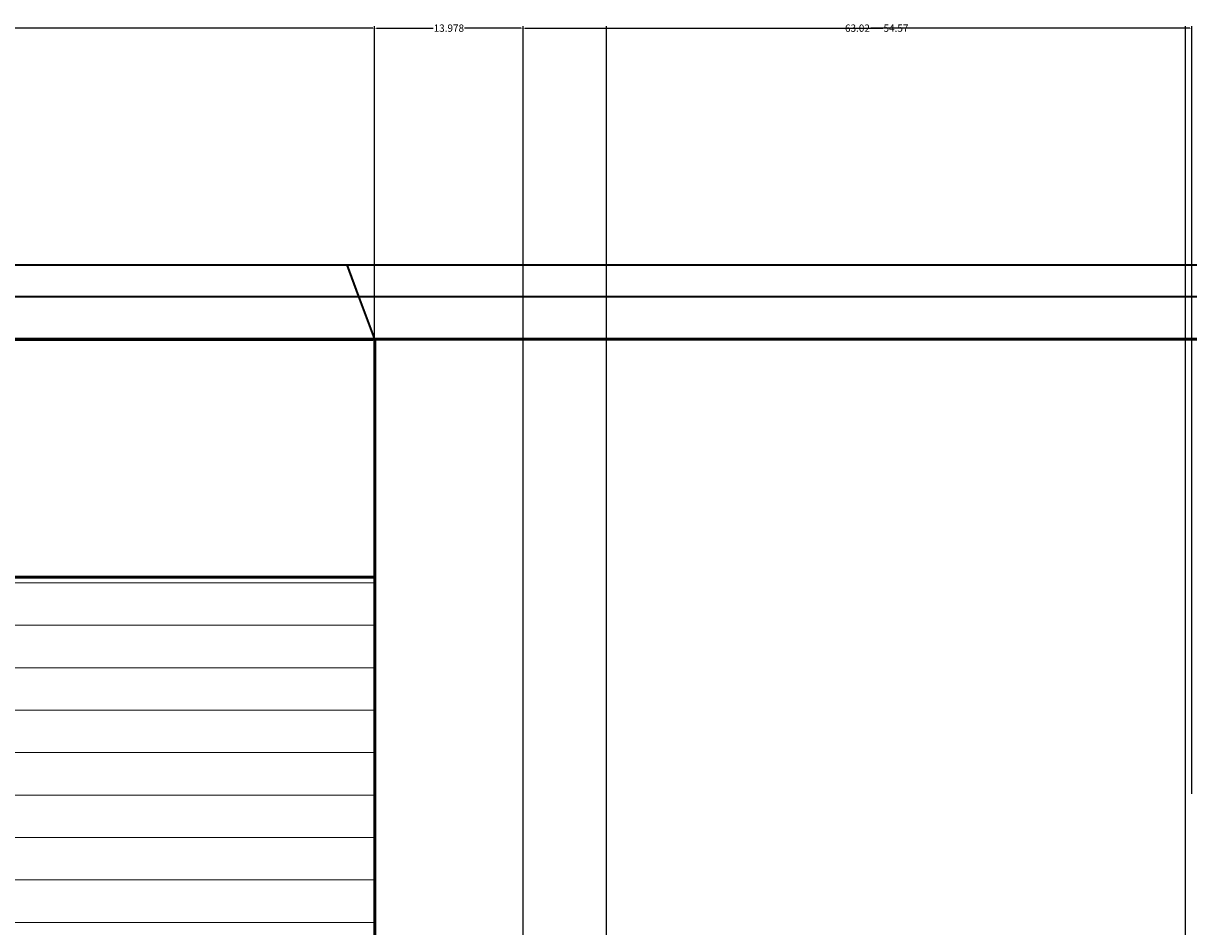
# Model space of a CAD drawing. Units: inches. Extents: x -139 to 346, y 72 to 413.
# Tile 10 of 18: x 66 to 175, y 328 to 413. Entities that reach past the tile are written whole.
import ezdxf

# ---------------------------------------------------------------- set-up
doc = ezdxf.new("R2010")
doc.units = ezdxf.units.IN
doc.header["$MEASUREMENT"] = 0
for name, color, linetype, lineweight in [('A-ANNO-DIMS', 2, 'Continuous', 18), ('A-ROOF', 1, 'Continuous', 35), ('A-WALL', 7, 'Continuous', 50), ('A-WALL-PATT', 8, 'Continuous', 13)]:
    doc.layers.add(name, color=color, linetype=linetype, lineweight=lineweight)
doc.styles.get("Standard").update_dxf_attribs({"font": 'arial.ttf'})
doc.dimstyles.get("Standard").update_dxf_attribs({"dimtxt": 0.6875, "dimasz": 0.18, "dimexe": 0.18, "dimexo": 0.0625, "dimgap": 0.09, "dimtad": 0, "dimtih": 1, "dimtoh": 1, "dimdec": 4, "dimzin": 0, "dimdsep": 46, "dimlunit": 4, "dimtxsty": 'Standard', "dimcen": 0.09, "dimadec": 0, "dimazin": 0, "dimtfac": 1, "dimtdec": 4, "dimtofl": 0, "dimtmove": 0, "dimatfit": 3, "dimfxl": 1, "dimtolj": 1, "dimtzin": 0, "dimarcsym": 0})

# ---------------------------------------------------------------- blocks, each defined once
blk = doc.blocks.new('*D25')
at = {"layer": 'A-ANNO-DIMS', "color": 0, "lineweight": -2, "transparency": 16777216}
for p, q in [((5.67, 338.38), (5.67, 412.45)), ((5.85, 412.27), (51.59, 412.27)), ((98.49, 412.27), (52.76, 412.27)), ((98.67, 360.61), (98.67, 412.45))]:
    blk.add_line(p, q, dxfattribs=at)
at = {"layer": 'A-ANNO-DIMS', "color": 0, "transparency": 16777216}
for points in [[(5.85, 412.3), (5.85, 412.24), (5.67, 412.27)], [(98.49, 412.3), (98.49, 412.24), (98.67, 412.27)]]:
    blk.add_solid(points, dxfattribs=at)
at = {"layer": 'Defpoints', "color": 0, "transparency": 16777216}
for p in [(98.67, 412.27), (98.67, 360.54), (5.67, 338.32)]:
    blk.add_point(p, dxfattribs=at)
at = {"layer": 'A-ANNO-DIMS', "color": 0, "transparency": 16777216, "insert": (52.17, 412.27), "char_height": 0.688, "attachment_point": 5}
blk.add_mtext('\\A1;93', dxfattribs=at)
blk = doc.blocks.new('*D26')
at = {"layer": 'A-ANNO-DIMS', "color": 0, "lineweight": -2, "transparency": 16777216}
for p, q in [((98.67, 360.61), (98.67, 412.45)), ((98.85, 412.27), (104.18, 412.27)), ((112.47, 412.27), (107.15, 412.27)), ((112.65, 291.12), (112.65, 412.45))]:
    blk.add_line(p, q, dxfattribs=at)
at = {"layer": 'A-ANNO-DIMS', "color": 0, "transparency": 16777216}
for points in [[(98.85, 412.3), (98.85, 412.24), (98.67, 412.27)], [(112.47, 412.3), (112.47, 412.24), (112.65, 412.27)]]:
    blk.add_solid(points, dxfattribs=at)
at = {"layer": 'Defpoints', "color": 0, "transparency": 16777216}
for p in [(112.65, 412.27), (98.67, 360.54), (112.65, 291.06)]:
    blk.add_point(p, dxfattribs=at)
at = {"layer": 'A-ANNO-DIMS', "color": 0, "transparency": 16777216, "insert": (105.66, 412.27), "char_height": 0.688, "attachment_point": 5}
blk.add_mtext('\\A1;13.978', dxfattribs=at)
blk = doc.blocks.new('*D27')
at = {"layer": 'A-ANNO-DIMS', "color": 0, "lineweight": -2, "transparency": 16777216}
for p, q in [((112.65, 291.12), (112.65, 412.45)), ((112.83, 412.27), (142.91, 412.27)), ((175.49, 412.27), (145.41, 412.27)), ((175.67, 340.12), (175.67, 412.45))]:
    blk.add_line(p, q, dxfattribs=at)
at = {"layer": 'A-ANNO-DIMS', "color": 0, "transparency": 16777216}
for points in [[(112.83, 412.3), (112.83, 412.24), (112.65, 412.27)], [(175.49, 412.3), (175.49, 412.24), (175.67, 412.27)]]:
    blk.add_solid(points, dxfattribs=at)
at = {"layer": 'Defpoints', "color": 0, "transparency": 16777216}
for p in [(175.67, 412.27), (175.67, 340.05), (112.65, 291.06)]:
    blk.add_point(p, dxfattribs=at)
at = {"layer": 'A-ANNO-DIMS', "color": 0, "transparency": 16777216, "insert": (144.16, 412.27), "char_height": 0.688, "attachment_point": 5}
blk.add_mtext('\\A1;63.02', dxfattribs=at)
blk = doc.blocks.new('*D30')
at = {"layer": 'A-ANNO-DIMS', "color": 0, "lineweight": -2, "transparency": 16777216}
for p, q in [((-34.73, 360.61), (-34.73, 383.02)), ((-34.55, 382.84), (30.75, 382.84)), ((98.49, 382.84), (33.19, 382.84)), ((98.67, 360.61), (98.67, 383.02))]:
    blk.add_line(p, q, dxfattribs=at)
at = {"layer": 'A-ANNO-DIMS', "color": 0, "transparency": 16777216}
for points in [[(-34.55, 382.87), (-34.55, 382.81), (-34.73, 382.84)], [(98.49, 382.87), (98.49, 382.81), (98.67, 382.84)]]:
    blk.add_solid(points, dxfattribs=at)
at = {"layer": 'Defpoints', "color": 0, "transparency": 16777216}
for p in [(98.67, 382.84), (-34.73, 360.54), (98.67, 360.54)]:
    blk.add_point(p, dxfattribs=at)
at = {"layer": 'A-ANNO-DIMS', "color": 0, "transparency": 16777216, "insert": (31.97, 382.84), "char_height": 0.688, "attachment_point": 5}
blk.add_mtext('\\A1;133.4', dxfattribs=at)
blk = doc.blocks.new('*D69')
at = {"layer": 'A-ANNO-DIMS', "color": 0, "lineweight": -2, "transparency": 16777216}
for p, q in [((120.51, 231.12), (120.51, 412.45)), ((120.69, 412.27), (146.54, 412.27)), ((174.89, 412.27), (149.04, 412.27)), ((175.07, 231.12), (175.07, 412.45))]:
    blk.add_line(p, q, dxfattribs=at)
at = {"layer": 'A-ANNO-DIMS', "color": 0, "transparency": 16777216}
for points in [[(120.69, 412.3), (120.69, 412.24), (120.51, 412.27)], [(174.89, 412.3), (174.89, 412.24), (175.07, 412.27)]]:
    blk.add_solid(points, dxfattribs=at)
at = {"layer": 'Defpoints', "color": 0, "transparency": 16777216}
for p in [(175.07, 412.27), (120.51, 231.06), (175.07, 231.06)]:
    blk.add_point(p, dxfattribs=at)
at = {"layer": 'A-ANNO-DIMS', "color": 0, "transparency": 16777216, "insert": (147.79, 412.27), "char_height": 0.688, "attachment_point": 5}
blk.add_mtext('\\A1;54.57', dxfattribs=at)

msp = doc.modelspace()

# ---------------------------------------------------------------- hatches: boundary and pattern name
at = {"layer": 'A-WALL-PATT'}
h = msp.add_hatch(dxfattribs=at)
h.set_pattern_fill('ANSI31', color=256, scale=32, angle=135)
h.paths.add_polyline_path([(98.6724, 360.5443), (-34.7346, 360.5443), (-34.7346, 353.0644), (-34.7346, 305.9205), (5.6729, 305.9205), (5.6729, 338.3217), (62.4258, 338.3217), (62.4258, 305.9205), (98.6724, 305.9205)])
h.paths.add_polyline_path([(212.769, 231.0607), (175.072, 231.0607), (175.072, 218.0635), (171.0337, 218.0635), (171.0337, 115.6761), (125.2464, 115.6761), (125.2464, 218.0635), (123.4318, 218.0635), (120.5054, 218.0635), (120.5054, 231.0607), (112.6506, 231.0607), (112.6506, 112.6042), (212.769, 112.6042)])

# ---------------------------------------------------------------- linework, layer by layer
at = {"layer": 'A-ROOF'}
for p, q in [((-47.2734, 389.9748), (309.8894, 389.9748)), ((97.189, 386.9748), (96.0765, 389.9748)), ((-47.2734, 386.9748), (309.8894, 386.9748)), ((98.6724, 382.9748), (97.189, 386.9748))]:
    msp.add_line(p, q, dxfattribs=at)
at = {"layer": 'A-WALL'}
for p, q in [((89.4597, 382.9748), (-47.2734, 382.9748)), ((309.8894, 382.9748), (89.4597, 382.9748)), ((98.6724, 305.9205), (98.6724, 382.9748)), ((-34.7346, 360.5443), (98.6724, 360.5443))]:
    msp.add_line(p, q, dxfattribs=at)

# ---------------------------------------------------------------- dimensions: what is measured, and where the dimension line sits
at = {"layer": 'A-ANNO-DIMS'}
for base, p1, p2, override, picture, middle in [((98.6724, 412.2748), (5.6729, 338.3217), (98.6724, 360.5443), {"dimdec": 0, "dimlfac": 1, "dimrnd": 0, "dimzin": 0, "dimdsep": 46, "dimlunit": 2}, '*D25', (52.1727, 412.2748)), ((112.6506, 412.2748), (98.6724, 360.5443), (112.6506, 291.0604), {"dimdec": 3, "dimlfac": 1, "dimrnd": 0, "dimzin": 0, "dimdsep": 46, "dimlunit": 2}, '*D26', (105.6615, 412.2748)), ((175.6676, 412.2748), (112.6506, 291.0604), (175.6676, 340.0548), {"dimdec": 2, "dimlfac": 1, "dimrnd": 0, "dimzin": 0, "dimdsep": 46, "dimlunit": 2}, '*D27', (144.1591, 412.2748)), ((175.072, 412.2748), (120.5054, 231.0607), (175.072, 231.0607), {"dimdec": 2, "dimlfac": 1, "dimrnd": 0, "dimzin": 0, "dimdsep": 46, "dimlunit": 2}, '*D69', (147.7887, 412.2748)), ((98.6724, 382.8443), (-34.7346, 360.5443), (98.6724, 360.5443), {"dimdec": 1, "dimlfac": 1, "dimrnd": 0, "dimzin": 0, "dimdsep": 46, "dimlunit": 2}, '*D30', (31.9689, 382.8443))]:
    dim = msp.add_linear_dim(base=base, p1=p1, p2=p2, dimstyle='Standard', override=override, dxfattribs=at)
    dim.commit()
    dim.dimension.update_dxf_attribs({"geometry": picture, "text_midpoint": middle})

doc.saveas('drawing.dxf')
